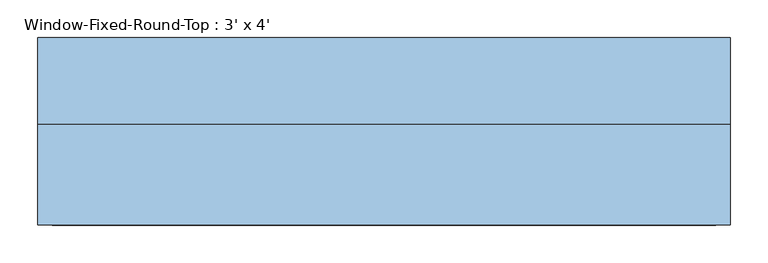
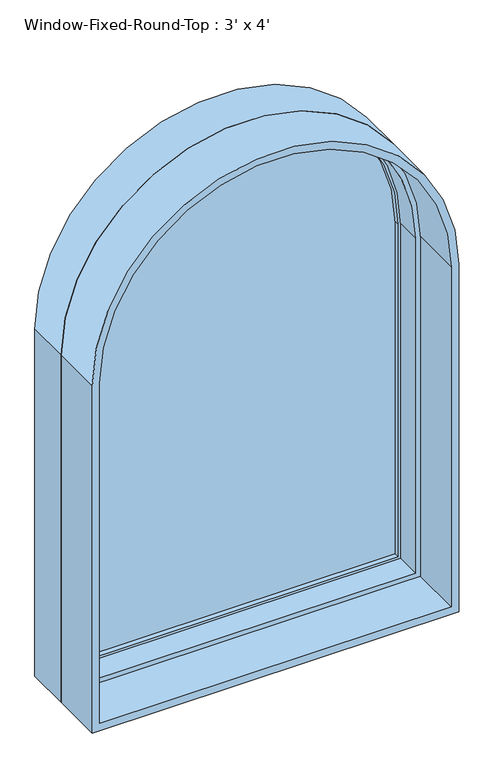
"""IFC4 building model written with IfcOpenShell, lengths in millimetres: window geometry, Window-Fixed-Round-Top : 3' x 4'."""

from ifc_helpers import new_model, si_unit, point, frame, frame_2d, origin, place, context, project, spatial, polyline, circle_curve, trimmed, segment, composite_curve, outline, extrude, source, transform, mapped, element, save
from ifc_brep_helpers import plane_surface, cylinder_surface, revolved_surface, advanced_brep


def window_fixed_round_top_3_x_4_dee2be1c(model_context):
    return source(origin(), model_context, "Body", "SolidModel", [
        advanced_brep(
        [(-425.45, 82.55, 1828.8), (-425.45, 19.05, 1828.8), (-425.45, 19.05, 946.15), (-425.45, 82.55, 946.15), (-444.5, 133.35, 1828.8), (-444.5, 82.55, 1828.8), (-444.5, 82.55, 927.1), (-444.5, 133.35, 927.1), (-457.2, 19.05, 1828.8), (-457.2, 133.35, 1828.8), (-457.2, 133.35, 914.4), (-457.2, 19.05, 914.4), (425.45, 19.05, 946.15), (425.45, 82.55, 946.15), (444.5, 82.55, 927.1), (444.5, 133.35, 927.1), (457.2, 133.35, 914.4), (457.2, 19.05, 914.4), (425.45, 19.05, 1828.8), (425.45, 82.55, 1828.8), (444.5, 82.55, 1828.8), (444.5, 133.35, 1828.8), (457.2, 133.35, 1828.8), (457.2, 19.05, 1828.8)],
        [
            (0, 1),
            (1, 2),
            (2, 3),
            (3, 0),
            (4, 5),
            (5, 6),
            (6, 7),
            (7, 4),
            (8, 9),
            (9, 10),
            (10, 11),
            (11, 8),
            (2, 12),
            (12, 13),
            (13, 3),
            (6, 14),
            (14, 15),
            (15, 7),
            (10, 16),
            (16, 17),
            (17, 11),
            (12, 18),
            (18, 19),
            (19, 13),
            (14, 20),
            (20, 21),
            (21, 15),
            (16, 22),
            (22, 23),
            (23, 17),
            (23, 8, circle_curve(frame((0.0, 19.05, 1828.8), z_axis=(0.0, -1.0, 0.0), x_axis=(1.0, 0.0, 0.0)), 457.2)),
            (1, 18, circle_curve(frame((0.0, 19.05, 1828.8), z_axis=(0.0, 1.0, 0.0), x_axis=(1.0, 0.0, 0.0)), 425.45)),
            (0, 19, circle_curve(frame((0.0, 82.55, 1828.8), z_axis=(0.0, 1.0, 0.0), x_axis=(1.0, 0.0, 0.0)), 425.45)),
            (5, 20, circle_curve(frame((0.0, 82.55, 1828.8), z_axis=(0.0, 1.0, 0.0), x_axis=(1.0, 0.0, 0.0)), 444.5)),
            (4, 21, circle_curve(frame((0.0, 133.35, 1828.8), z_axis=(0.0, 1.0, 0.0), x_axis=(1.0, 0.0, 0.0)), 444.5)),
            (9, 22, circle_curve(frame((0.0, 133.35, 1828.8), z_axis=(0.0, 1.0, 0.0), x_axis=(1.0, 0.0, 0.0)), 457.2)),
        ],
        [
            plane_surface(frame((-425.45, 19.05, 1828.8), z_axis=(1.0, 0.0, 0.0), x_axis=(0.0, 0.0, -1.0))),
            plane_surface(frame((-444.5, 82.55, 1828.8), z_axis=(1.0, 0.0, 0.0), x_axis=(0.0, 0.0, -1.0))),
            plane_surface(frame((-457.2, 133.35, 1828.8), z_axis=(-1.0, 0.0, 0.0), x_axis=(0.0, 0.0, -1.0))),
            plane_surface(frame((-425.45, 19.05, 946.15), z_axis=(0.0, 0.0, 1.0), x_axis=(1.0, 0.0, 0.0))),
            plane_surface(frame((-444.5, 82.55, 927.1), z_axis=(0.0, 0.0, 1.0), x_axis=(1.0, 0.0, 0.0))),
            plane_surface(frame((-457.2, 133.35, 914.4), z_axis=(0.0, 0.0, -1.0), x_axis=(1.0, 0.0, 0.0))),
            plane_surface(frame((425.45, 19.05, 946.15), z_axis=(-1.0, 0.0, 0.0), x_axis=(0.0, 0.0, 1.0))),
            plane_surface(frame((444.5, 82.55, 927.1), z_axis=(-1.0, 0.0, 0.0), x_axis=(0.0, 0.0, 1.0))),
            plane_surface(frame((457.2, 133.35, 914.4), z_axis=(1.0, 0.0, 0.0), x_axis=(0.0, 0.0, 1.0))),
            plane_surface(frame((0.0, 19.05, 1828.8), z_axis=(0.0, -1.0, 0.0), x_axis=(1.0, 0.0, 0.0))),
            revolved_surface(polyline([(425.45, 19.049999999999997, 1828.8), (425.45, 82.55, 1828.8)]), (0.0, 127.0, 1828.8), (0.0, -1.0, 0.0)),
            plane_surface(frame((0.0, 82.55, 1828.8), z_axis=(0.0, 1.0, 0.0), x_axis=(1.0, 0.0, 0.0))),
            revolved_surface(polyline([(444.5, 82.55, 1828.8), (444.5, 133.35, 1828.8)]), (0.0, 127.0, 1828.8), (0.0, -1.0, 0.0)),
            plane_surface(frame((0.0, 133.35, 1828.8), z_axis=(0.0, 1.0, 0.0), x_axis=(1.0, 0.0, 0.0))),
            cylinder_surface(frame((0.0, 127.0, 1828.8), z_axis=(0.0, -1.0, 0.0), x_axis=(1.0, 0.0, 0.0)), 457.2),
        ],
        [
            (0, [[1, 2, 3, 4]]),
            (1, [[5, 6, 7, 8]]),
            (2, [[9, 10, 11, 12]]),
            (3, [[-3, 13, 14, 15]]),
            (4, [[-7, 16, 17, 18]]),
            (5, [[-11, 19, 20, 21]]),
            (6, [[-14, 22, 23, 24]]),
            (7, [[-17, 25, 26, 27]]),
            (8, [[-20, 28, 29, 30]]),
            (9, [[-21, -30, 31, -12], [32, -22, -13, -2]]),
            (10, [[33, -23, -32, -1]]),
            (11, [[34, -25, -16, -6], [-15, -24, -33, -4]]),
            (12, [[35, -26, -34, -5]]),
            (13, [[36, -28, -19, -10], [-18, -27, -35, -8]]),
            (14, [[-31, -29, -36, -9]]),
        ],
    ),
        extrude(outline(composite_curve([segment(trimmed(circle_curve(frame_2d((1828.8, 0.0)), 457.2), [point((1828.8, 457.2))], [point((1828.8, -457.2))], False, "CARTESIAN"), True, "CONTINUOUS"), segment(polyline([(1828.8, -457.2), (914.4, -457.2), (914.4, 457.2), (1828.8, 457.2)]), True, "CONTINUOUS")], self_intersect=False), holes=[composite_curve([segment(polyline([(1828.8, 438.15), (933.45, 438.15), (933.45, -438.15), (1828.8, -438.15)]), True, "CONTINUOUS"), segment(trimmed(circle_curve(frame_2d((1828.8, 0.0)), 438.15), [point((1828.8, -438.15))], [point((1828.8, 438.15))], True, "CARTESIAN"), True, "CONTINUOUS")], self_intersect=False)]), frame((0.0, -114.3, 0.0), z_axis=(0.0, 1.0, 0.0), x_axis=(0.0, 0.0, 1.0)), (0.0, 0.0, 1.0), 133.35),
        extrude(outline(composite_curve([segment(polyline([(927.1, 444.5), (1828.8, 444.5)]), True, "CONTINUOUS"), segment(trimmed(circle_curve(frame_2d((1828.8, 0.0)), 444.5), [point((1828.8, 444.5))], [point((1828.8, -444.5))], False, "CARTESIAN"), True, "CONTINUOUS"), segment(polyline([(1828.8, -444.5), (927.1, -444.5), (927.1, 444.5)]), True, "CONTINUOUS")], self_intersect=False), holes=[composite_curve([segment(polyline([(952.5, -419.1), (1828.8, -419.1)]), True, "CONTINUOUS"), segment(trimmed(circle_curve(frame_2d((1828.8, 0.0)), 419.1), [point((1828.8, -419.1))], [point((1828.8, 419.1))], True, "CARTESIAN"), True, "CONTINUOUS"), segment(polyline([(1828.8, 419.1), (952.5, 419.1), (952.5, -419.1)]), True, "CONTINUOUS")], self_intersect=False)]), frame((0.0, 82.55, 0.0), z_axis=(0.0, 1.0, 0.0), x_axis=(0.0, 0.0, 1.0)), (0.0, 0.0, 1.0), 31.75),
        extrude(outline(composite_curve([segment(trimmed(circle_curve(frame_2d((1828.8, 0.0)), 419.1), [point((1828.8, 419.1))], [point((1828.8, -419.1))], False, "CARTESIAN"), True, "CONTINUOUS"), segment(polyline([(1828.8, -419.1), (952.5, -419.1), (952.5, 419.1), (1828.8, 419.1)]), True, "CONTINUOUS")], self_intersect=False)), frame((0.0, 107.95, 0.0), z_axis=(0.0, 1.0, 0.0), x_axis=(0.0, 0.0, 1.0)), (0.0, 0.0, 1.0), 6.35),
        extrude(outline(composite_curve([segment(trimmed(circle_curve(frame_2d((1828.8, 0.0)), 419.1), [point((1828.8, 419.1))], [point((1828.8, -419.1))], False, "CARTESIAN"), True, "CONTINUOUS"), segment(polyline([(1828.8, -419.1), (952.5, -419.1), (952.5, 419.1), (1828.8, 419.1)]), True, "CONTINUOUS")], self_intersect=False)), frame((0.0, 95.25, 0.0), z_axis=(0.0, 1.0, 0.0), x_axis=(0.0, 0.0, 1.0)), (0.0, 0.0, 1.0), 6.35),
        extrude(outline(composite_curve([segment(polyline([(1828.8, -444.5), (927.1, -444.5), (927.1, 444.5), (1828.8, 444.5)]), True, "CONTINUOUS"), segment(trimmed(circle_curve(frame_2d((1828.8, 0.0)), 444.5), [point((1828.8, 444.5))], [point((1828.8, -444.5))], False, "CARTESIAN"), True, "CONTINUOUS")], self_intersect=False), holes=[composite_curve([segment(polyline([(1828.8, 419.1), (952.5, 419.1), (952.5, -419.1), (1828.8, -419.1)]), True, "CONTINUOUS"), segment(trimmed(circle_curve(frame_2d((1828.8, 0.0)), 419.1), [point((1828.8, -419.1))], [point((1828.8, 419.1))], True, "CARTESIAN"), True, "CONTINUOUS")], self_intersect=False)]), frame((0.0, 114.3, 0.0), z_axis=(0.0, 1.0, 0.0), x_axis=(0.0, 0.0, 1.0)), (0.0, 0.0, 1.0), 12.7),
    ])


if __name__ == "__main__":
    model = new_model("IFC4")
    model_context = context("Model", 3, world=origin())
    ifc_project = project(units=[si_unit("LENGTHUNIT", "METRE", prefix="MILLI")], contexts=[model_context])
    site = spatial("IfcSite", under=ifc_project)
    building = spatial("IfcBuilding", under=site)
    placement = place(None, origin())
    window_fixed_round_top_3_x_4_shape = window_fixed_round_top_3_x_4_dee2be1c(model_context)
    element("IfcWindow", 1, ObjectType="Window-Fixed-Round-Top : 3' x 4'", at=placement, inside=building, context=model_context, shape_type="MappedRepresentation", body=[
        mapped(window_fixed_round_top_3_x_4_shape, transform((0.0, 0.0, 0.0), x_axis=(1.0, 0.0, 0.0), y_axis=(0.0, 1.0, 0.0), z_axis=(0.0, 0.0, 1.0))),
    ])
    save(model, "model.ifc")

# Revit data of these elements
# Type "Window-Fixed-Round-Top : 3' x 4'"
#   Type Mark = "21"
#   Fire Rating = "0.5h"
#   Assembly Code = "B2020100"
#   Analytic Construction = "Double glazing - domestic"
#   Window Inset [instance default] = 0' - 0"
#   Wall Thickness [instance default] = 0' - 6"
#   Visual Light Transmittance = 0.81
#   Thermal Resistance (R) = 1.8146 (h·ft²·°F)/BTU
#   Solar Heat Gain Coefficient = 0.76
#   Rough Width = 3' - 0 1/2"
#   Rough Height = 4' - 6 1/2"
#   Interior Wall Closure [instance default] = 0' - 2 1/4"
#   Height = 4' - 6"
#   Heat Transfer Coefficient (U) = 0.5511 BTU/(h·ft²·°F)
#   Frame Extension [instance default] = 0' - 0 1/4"
#   Exterior Wall Closure [instance default] = 0' - 1 1/4"
#   Extension Jamb [instance default] = 0' - 2 1/4"
#   Default Sill Height = 3' - 0"
#   Width = 3' - 0"
#   Interior Trim Visibility [instance default] = yes
#   Exterior Trim Visibility [instance default] = yes
#   Extension Jamb Visibility [instance default] = yes
#   Interior Trim Material = Wood - Stained
#   Interior Trim = Trim-Window-Interior-Flat-Arch-Top-Tree_Centered : Picture Frame
#   Interior Frame Material = Wood - Stained
#   Glass Panel Material = Glass
#   Exterior Trim Material = Clad - White
#   Exterior Trim = Trim-Window-Exterior-Flat-Arch-Top-Tree_Centered : with Sill
#   Exterior Frame Material = Clad - White
#   Wall Closure = (empty or 0)
# Element 1 (IfcWindow, "Window-Fixed-Round-Top : 3' x 4'")
#   Wall Thickness = 0' - 9"
#   Extension Jamb = 0' - 5 1/4"
#   Materials on its faces: "Wood - Stained", "Clad - White", "Glass"
# Materials
#   "Wood - Stained": class "Wood", colour RGB 224 178 126, transparency 0, Cost = 0
#   "Glass": class "Glass", colour RGB 0 128 192, transparency 0.75, Description = "Soda Lime Glass", Cost = 0
#   "Clad - White": class "Wood", colour RGB 242 242 238, transparency 0, Cost = 0
